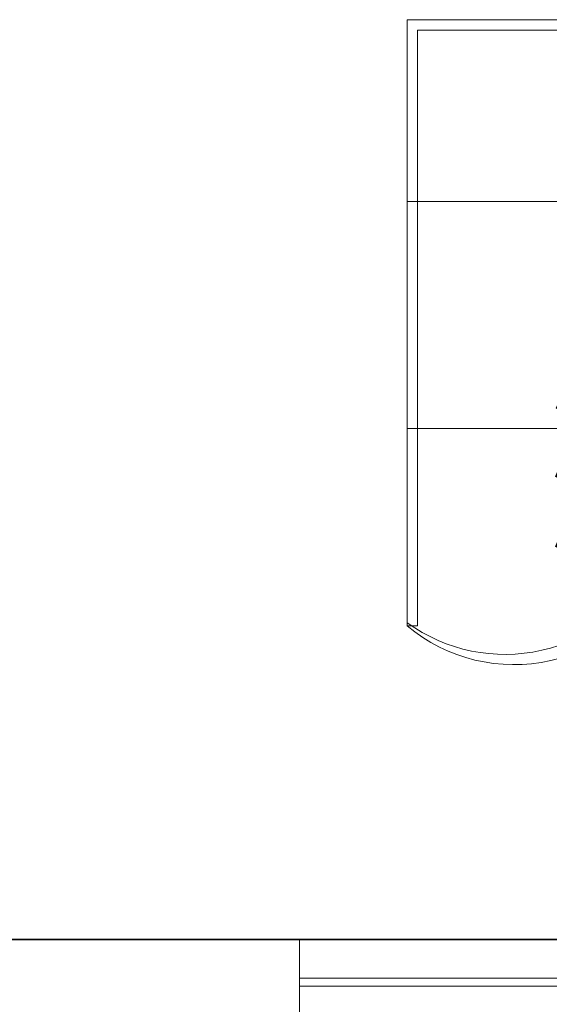
# Model space of a CAD drawing. Units: inches. Extents: x -61 to 1599, y -1316 to 257.
# Tile 159 of 204: x 1163 to 1214, y -1208 to -1113. Entities that reach past the tile are written whole.
import ezdxf

# ---------------------------------------------------------------- set-up
doc = ezdxf.new("R2010")
doc.units = ezdxf.units.IN
doc.header["$MEASUREMENT"] = 0
for name, color, linetype, lineweight in [('FURNITURE', 83, 'Continuous', 18), ('WALLS', 4, 'Continuous', 35), ('WINDOWS', 220, 'Continuous', 18)]:
    doc.layers.add(name, color=color, linetype=linetype, lineweight=lineweight)

# ---------------------------------------------------------------- blocks, each defined once
blk = doc.blocks.new('WIN-36IN-2')
for p, q in [((0, 9), (0, 0)), ((36, 9), (36, 0)), ((0, 5.262), (36, 5.262)), ((0, 4.5), (36, 4.5)), ((0, 4.5), (36, 4.5))]:
    blk.add_line(p, q)
blk = doc.blocks.new('MASTER-BEDROOM-CONSOLE')
for p, q in [((0, 44.886), (23.587, 44.886)), ((23.587, 37.779), (23.587, 9.438)), ((23.587, 37.779), (24.943, 35.589)), ((24.943, 35.589), (24.943, 9.456)), ((18.162, 33.228), (18.879, 30.704)), ((18.162, 33.228), (19.133, 31.826)), ((18.162, 33.228), (18.181, 31.167)), ((23.587, 30.804), (21.228, 29.654)), ((23.587, 30.804), (21.894, 30.592)), ((23.587, 30.804), (22.038, 29.443)), ((18.203, 28.51), (18.441, 28.869)), ((18.441, 28.869), (18.678, 29.228)), ((19.963, 28.553), (19.841, 28.966)), ((19.008, 27.84), (18.615, 28.016)), ((19.008, 27.84), (18.707, 27.533)), ((19.008, 27.84), (18.833, 27.448)), ((19.008, 27.84), (18.886, 28.253)), ((19.184, 28.233), (19.008, 27.84)), ((19.309, 28.148), (19.008, 27.84)), ((19.401, 27.665), (19.008, 27.84)), ((19.13, 27.428), (19.008, 27.84)), ((20.085, 28.141), (19.963, 28.553)), ((18.061, 27.072), (17.939, 27.485)), ((18.183, 26.66), (18.061, 27.072)), ((19.38, 26.517), (19.618, 26.876)), ((19.618, 26.876), (19.855, 27.235)), ((14.429, 24.877), (15.978, 26.238)), ((14.429, 24.877), (16.788, 26.026)), ((18.084, 26.588), (18.801, 24.064)), ((18.084, 26.588), (19.055, 25.186)), ((18.084, 26.588), (18.103, 24.527)), ((14.429, 24.877), (16.122, 25.089)), ((19.854, 22.452), (19.137, 24.976)), ((19.854, 22.452), (19.835, 24.514)), ((23.509, 24.163), (21.15, 23.014)), ((23.509, 24.163), (21.816, 23.952)), ((23.509, 24.163), (21.96, 22.803)), ((19.854, 22.452), (18.883, 23.854)), ((0, 22.886), (23.587, 22.886)), ((18.125, 21.87), (18.362, 22.229)), ((18.362, 22.229), (18.6, 22.588)), ((19.885, 21.913), (19.763, 22.326)), ((18.93, 21.2), (18.537, 21.376)), ((18.93, 21.2), (18.629, 20.893)), ((18.93, 21.2), (18.754, 20.808)), ((18.93, 21.2), (18.808, 21.613)), ((19.105, 21.593), (18.93, 21.2)), ((19.23, 21.508), (18.93, 21.2)), ((19.322, 21.025), (18.93, 21.2)), ((19.052, 20.788), (18.93, 21.2)), ((20.007, 21.5), (19.885, 21.913)), ((17.983, 20.432), (17.861, 20.845)), ((18.105, 20.02), (17.983, 20.432)), ((19.302, 19.877), (19.54, 20.236)), ((19.54, 20.236), (19.777, 20.595)), ((14.351, 18.237), (15.9, 19.598)), ((14.351, 18.237), (16.71, 19.386)), ((18.084, 19.819), (18.801, 17.295)), ((18.084, 19.819), (19.055, 18.417)), ((18.084, 19.819), (18.103, 17.757)), ((14.351, 18.237), (16.043, 18.448)), ((19.776, 15.812), (19.059, 18.336)), ((19.776, 15.812), (18.804, 17.214)), ((19.776, 15.812), (19.757, 17.874)), ((23.509, 17.394), (21.15, 16.245)), ((23.509, 17.394), (21.816, 17.183)), ((23.509, 17.394), (21.96, 16.033)), ((18.125, 15.101), (18.362, 15.459)), ((18.362, 15.459), (18.6, 15.818)), ((19.885, 15.143), (19.763, 15.556)), ((18.93, 14.431), (18.537, 14.606)), ((18.93, 14.431), (18.629, 14.123)), ((18.93, 14.431), (18.754, 14.038)), ((18.93, 14.431), (18.808, 14.843)), ((19.105, 14.823), (18.93, 14.431)), ((19.23, 14.738), (18.93, 14.431)), ((19.322, 14.255), (18.93, 14.431)), ((19.052, 14.018), (18.93, 14.431)), ((20.007, 14.731), (19.885, 15.143)), ((17.983, 13.663), (17.861, 14.075)), ((18.105, 13.25), (17.983, 13.663)), ((19.302, 13.108), (19.54, 13.466)), ((19.54, 13.466), (19.777, 13.825)), ((14.351, 11.468), (15.9, 12.828)), ((14.351, 11.468), (16.71, 12.617)), ((14.351, 11.468), (16.043, 11.679)), ((19.776, 9.043), (19.059, 11.567)), ((19.776, 9.043), (19.757, 11.104)), ((19.776, 9.043), (18.804, 10.445)), ((22.587, 9.438), (23.587, 9.438)), ((1, 3.748), (0, 3.748))]:
    blk.add_line(p, q)
for points in [[(0, 3.748), (0, 62.524), (23.587, 62.524), (23.587, 9.438)], [(1, 3.748), (1, 61.524), (22.587, 61.524), (22.587, 9.438)]]:
    blk.add_lwpolyline(points)
for points in [[(14.429, 24.877), (18.162, 33.228), (23.587, 30.804), (19.854, 22.452)], [(14.351, 18.237), (18.084, 26.588), (23.509, 24.163), (19.776, 15.812)], [(14.351, 11.468), (18.084, 19.819), (23.509, 17.394), (19.776, 9.043)]]:
    blk.add_lwpolyline(points, close=True)
for centre, radius in [((19.008, 27.84), 0.567), ((19.008, 27.84), 0.567), ((19.008, 27.84), 0.43), ((18.93, 21.2), 0.567), ((18.93, 21.2), 0.567), ((18.93, 21.2), 0.43), ((18.93, 14.431), 0.567), ((18.93, 14.431), 0.567), ((18.93, 14.431), 0.43)]:
    blk.add_circle(centre, radius)
for centre, radius, start, end in [((0.46, 36.131), 17.938, 321.14464, 350.6879), ((24.495, 40.115), 9.356, 227.40134, 264.43121), ((19.167, 31.62), 0.209, 99.3213, 167.2974), ((18.925, 31.877), 0.214, 280.21251, 346.40619), ((19.095, 32.037), 0.214, 280.21251, 346.40619), ((19.338, 31.78), 0.209, 99.3213, 167.2974), ((18.215, 30.96), 0.209, 99.3213, 167.2974), ((17.973, 31.217), 0.214, 280.21251, 346.40619), ((18.143, 31.378), 0.214, 280.21251, 346.40619), ((18.385, 31.121), 0.209, 99.3213, 167.2974), ((18.913, 30.498), 0.209, 99.3213, 167.2974), ((18.67, 30.755), 0.214, 280.21251, 346.40619), ((18.841, 30.915), 0.214, 280.21251, 346.40619), ((19.083, 30.658), 0.209, 99.3213, 167.2974), ((37.556, 19.55), 17.938, 141.14464, 170.6879), ((22.071, 30.471), 0.214, 145.42636, 211.62004), ((22.077, 30.705), 0.214, 145.42636, 211.62004), ((21.718, 30.48), 0.209, 324.53515, 32.51125), ((21.724, 30.714), 0.209, 324.53515, 32.51125), ((21.405, 29.533), 0.214, 145.42636, 211.62004), ((21.411, 29.767), 0.214, 145.42636, 211.62004), ((21.052, 29.542), 0.209, 324.53515, 32.51125), ((21.058, 29.776), 0.209, 324.53515, 32.51125), ((22.221, 29.555), 0.214, 145.42636, 211.62004), ((21.867, 29.564), 0.209, 324.53515, 32.51125), ((22.215, 29.321), 0.214, 145.42636, 211.62004), ((21.861, 29.33), 0.209, 324.53515, 32.51125), ((0.382, 29.491), 17.938, 321.14464, 350.6879), ((16.149, 26.117), 0.209, 144.53515, 212.51125), ((16.155, 26.351), 0.209, 144.53515, 212.51125), ((15.796, 26.126), 0.214, 325.42636, 31.62004), ((15.802, 26.36), 0.214, 325.42636, 31.62004), ((16.959, 25.905), 0.209, 144.53515, 212.51125), ((16.965, 26.139), 0.209, 144.53515, 212.51125), ((16.605, 25.914), 0.214, 325.42636, 31.62004), ((16.611, 26.148), 0.214, 325.42636, 31.62004), ((24.416, 33.475), 9.356, 227.40134, 264.43121), ((13.521, 15.565), 9.356, 47.40134, 84.43121), ((16.292, 24.967), 0.209, 144.53515, 212.51125), ((16.298, 25.201), 0.209, 144.53515, 212.51125), ((15.939, 24.976), 0.214, 325.42636, 31.62004), ((15.945, 25.21), 0.214, 325.42636, 31.62004), ((19.089, 24.98), 0.209, 99.3213, 167.2974), ((18.847, 25.237), 0.214, 280.21251, 346.40619), ((19.175, 24.765), 0.214, 100.21251, 166.40619), ((18.933, 25.022), 0.209, 279.3213, 347.2974), ((19.017, 25.397), 0.214, 280.21251, 346.40619), ((19.259, 25.14), 0.209, 99.3213, 167.2974), ((19.103, 25.183), 0.209, 279.3213, 347.2974), ((19.346, 24.926), 0.214, 100.21251, 166.40619), ((18.137, 24.32), 0.209, 99.3213, 167.2974), ((17.894, 24.577), 0.214, 280.21251, 346.40619), ((18.065, 24.738), 0.214, 280.21251, 346.40619), ((18.307, 24.48), 0.209, 99.3213, 167.2974), ((18.834, 23.858), 0.209, 99.3213, 167.2974), ((18.592, 24.115), 0.214, 280.21251, 346.40619), ((18.763, 24.275), 0.214, 280.21251, 346.40619), ((19.005, 24.018), 0.209, 99.3213, 167.2974), ((18.849, 24.061), 0.209, 279.3213, 347.2974), ((19.091, 23.804), 0.214, 100.21251, 166.40619), ((19.873, 24.303), 0.214, 100.21251, 166.40619), ((19.631, 24.56), 0.209, 279.3213, 347.2974), ((37.478, 12.91), 17.938, 141.14464, 170.6879), ((19.801, 24.721), 0.209, 279.3213, 347.2974), ((20.043, 24.464), 0.214, 100.21251, 166.40619), ((21.993, 23.83), 0.214, 145.42636, 211.62004), ((21.999, 24.065), 0.214, 145.42636, 211.62004), ((21.64, 23.84), 0.209, 324.53515, 32.51125), ((21.646, 24.074), 0.209, 324.53515, 32.51125), ((18.921, 23.643), 0.214, 100.21251, 166.40619), ((18.678, 23.9), 0.209, 279.3213, 347.2974), ((21.326, 22.892), 0.214, 145.42636, 211.62004), ((21.332, 23.127), 0.214, 145.42636, 211.62004), ((20.973, 22.902), 0.209, 324.53515, 32.51125), ((20.979, 23.136), 0.209, 324.53515, 32.51125), ((22.142, 22.915), 0.214, 145.42636, 211.62004), ((21.789, 22.924), 0.209, 324.53515, 32.51125), ((22.136, 22.681), 0.214, 145.42636, 211.62004), ((21.783, 22.69), 0.209, 324.53515, 32.51125), ((0.382, 22.721), 17.938, 321.14464, 350.6879), ((16.07, 19.476), 0.209, 144.53515, 212.51125), ((16.076, 19.711), 0.209, 144.53515, 212.51125), ((15.717, 19.486), 0.214, 325.42636, 31.62004), ((15.723, 19.72), 0.214, 325.42636, 31.62004), ((16.88, 19.265), 0.209, 144.53515, 212.51125), ((16.886, 19.499), 0.209, 144.53515, 212.51125), ((16.527, 19.274), 0.214, 325.42636, 31.62004), ((16.533, 19.508), 0.214, 325.42636, 31.62004), ((24.416, 26.706), 9.356, 227.40134, 264.43121), ((13.443, 8.925), 9.356, 47.40134, 84.43121), ((16.214, 18.327), 0.209, 144.53515, 212.51125), ((16.22, 18.561), 0.209, 144.53515, 212.51125), ((15.861, 18.336), 0.214, 325.42636, 31.62004), ((15.867, 18.57), 0.214, 325.42636, 31.62004), ((19.089, 18.21), 0.209, 99.3213, 167.2974), ((18.847, 18.467), 0.214, 280.21251, 346.40619), ((19.097, 18.125), 0.214, 100.21251, 166.40619), ((18.855, 18.382), 0.209, 279.3213, 347.2974), ((19.017, 18.628), 0.214, 280.21251, 346.40619), ((19.259, 18.371), 0.209, 99.3213, 167.2974), ((19.025, 18.543), 0.209, 279.3213, 347.2974), ((19.267, 18.286), 0.214, 100.21251, 166.40619), ((18.137, 17.55), 0.209, 99.3213, 167.2974), ((17.894, 17.807), 0.214, 280.21251, 346.40619), ((18.065, 17.968), 0.214, 280.21251, 346.40619), ((18.307, 17.711), 0.209, 99.3213, 167.2974), ((18.834, 17.088), 0.209, 99.3213, 167.2974), ((18.592, 17.345), 0.214, 280.21251, 346.40619), ((18.842, 17.003), 0.214, 100.21251, 166.40619), ((18.6, 17.26), 0.209, 279.3213, 347.2974), ((18.763, 17.506), 0.214, 280.21251, 346.40619), ((19.005, 17.249), 0.209, 99.3213, 167.2974), ((18.771, 17.421), 0.209, 279.3213, 347.2974), ((19.013, 17.164), 0.214, 100.21251, 166.40619), ((19.795, 17.663), 0.214, 100.21251, 166.40619), ((19.552, 17.92), 0.209, 279.3213, 347.2974), ((19.723, 18.081), 0.209, 279.3213, 347.2974), ((19.965, 17.824), 0.214, 100.21251, 166.40619), ((37.478, 6.14), 17.938, 141.14464, 170.6879), ((21.993, 17.061), 0.214, 145.42636, 211.62004), ((21.999, 17.295), 0.214, 145.42636, 211.62004), ((21.64, 17.07), 0.209, 324.53515, 32.51125), ((21.646, 17.304), 0.209, 324.53515, 32.51125), ((21.326, 16.123), 0.214, 145.42636, 211.62004), ((21.332, 16.357), 0.214, 145.42636, 211.62004), ((20.973, 16.132), 0.209, 324.53515, 32.51125), ((20.979, 16.366), 0.209, 324.53515, 32.51125), ((22.142, 16.145), 0.214, 145.42636, 211.62004), ((21.789, 16.155), 0.209, 324.53515, 32.51125), ((22.136, 15.911), 0.214, 145.42636, 211.62004), ((21.783, 15.92), 0.209, 324.53515, 32.51125), ((16.07, 12.707), 0.209, 144.53515, 212.51125), ((16.076, 12.941), 0.209, 144.53515, 212.51125), ((15.717, 12.716), 0.214, 325.42636, 31.62004), ((15.723, 12.95), 0.214, 325.42636, 31.62004), ((16.88, 12.495), 0.209, 144.53515, 212.51125), ((16.886, 12.729), 0.209, 144.53515, 212.51125), ((16.527, 12.504), 0.214, 325.42636, 31.62004), ((16.533, 12.739), 0.214, 325.42636, 31.62004), ((13.443, 2.156), 9.356, 47.40134, 84.43121), ((16.214, 11.557), 0.209, 144.53515, 212.51125), ((16.22, 11.791), 0.209, 144.53515, 212.51125), ((15.861, 11.566), 0.214, 325.42636, 31.62004), ((15.867, 11.801), 0.214, 325.42636, 31.62004), ((19.097, 11.356), 0.214, 100.21251, 166.40619), ((18.855, 11.613), 0.209, 279.3213, 347.2974), ((19.025, 11.773), 0.209, 279.3213, 347.2974), ((19.267, 11.516), 0.214, 100.21251, 166.40619), ((18.771, 10.651), 0.209, 279.3213, 347.2974), ((19.013, 10.394), 0.214, 100.21251, 166.40619), ((19.795, 10.893), 0.214, 100.21251, 166.40619), ((19.552, 11.151), 0.209, 279.3213, 347.2974), ((19.723, 11.311), 0.209, 279.3213, 347.2974), ((19.965, 11.054), 0.214, 100.21251, 166.40619), ((18.842, 10.234), 0.214, 100.21251, 166.40619), ((18.6, 10.491), 0.209, 279.3213, 347.2974), ((10.308, 16.053), 16.053, 230.04489, 335.73444), ((9.449, 17.042), 16.053, 233.93821, 331.72641)]:
    blk.add_arc(centre, radius, start, end)
for points in [[(18.203, 28.51), (18.191, 28.604), (18.167, 28.791), (18.438, 28.884), (18.778, 28.897), (18.67, 29.157), (18.678, 29.228)], [(20.085, 28.141), (20.124, 28.226), (20.202, 28.398), (19.97, 28.566), (19.649, 28.679), (19.829, 28.896), (19.841, 28.966)], [(19.401, 27.665), (19.361, 27.75), (19.281, 27.921), (19.003, 27.854), (18.708, 27.683), (18.66, 27.961), (18.615, 28.016)], [(19.309, 28.148), (19.303, 28.054), (19.292, 27.866), (19.008, 27.825), (18.671, 27.876), (18.729, 27.6), (18.707, 27.533)], [(19.13, 27.428), (19.169, 27.514), (19.247, 27.685), (19.015, 27.854), (18.694, 27.966), (18.873, 28.183), (18.886, 28.253)], [(19.184, 28.233), (19.098, 28.193), (18.927, 28.113), (18.994, 27.835), (19.165, 27.54), (18.888, 27.492), (18.833, 27.448)], [(18.183, 26.66), (18.222, 26.746), (18.3, 26.917), (18.069, 27.086), (17.747, 27.198), (17.927, 27.415), (17.939, 27.485)], [(19.38, 26.517), (19.368, 26.611), (19.344, 26.798), (19.615, 26.891), (19.955, 26.904), (19.847, 27.164), (19.855, 27.235)], [(18.125, 21.87), (18.113, 21.964), (18.089, 22.151), (18.359, 22.244), (18.7, 22.257), (18.592, 22.517), (18.6, 22.588)], [(20.007, 21.5), (20.046, 21.586), (20.124, 21.758), (19.892, 21.926), (19.571, 22.039), (19.75, 22.256), (19.763, 22.326)], [(19.322, 21.025), (19.283, 21.11), (19.203, 21.281), (18.924, 21.214), (18.63, 21.043), (18.582, 21.321), (18.537, 21.376)], [(19.23, 21.508), (19.225, 21.414), (19.213, 21.226), (18.93, 21.185), (18.593, 21.236), (18.651, 20.96), (18.629, 20.893)], [(19.052, 20.788), (19.091, 20.874), (19.169, 21.045), (18.937, 21.214), (18.615, 21.326), (18.795, 21.543), (18.808, 21.613)], [(19.105, 21.593), (19.02, 21.553), (18.849, 21.473), (18.916, 21.195), (19.087, 20.9), (18.809, 20.852), (18.754, 20.808)], [(18.105, 20.02), (18.144, 20.105), (18.222, 20.277), (17.99, 20.445), (17.669, 20.558), (17.848, 20.775), (17.861, 20.845)], [(19.302, 19.877), (19.29, 19.971), (19.266, 20.158), (19.537, 20.251), (19.877, 20.264), (19.769, 20.524), (19.777, 20.595)], [(18.125, 15.101), (18.113, 15.194), (18.089, 15.381), (18.359, 15.474), (18.7, 15.488), (18.592, 15.748), (18.6, 15.818)], [(20.007, 14.731), (20.046, 14.817), (20.124, 14.988), (19.892, 15.157), (19.571, 15.269), (19.75, 15.486), (19.763, 15.556)], [(19.322, 14.255), (19.283, 14.341), (19.203, 14.511), (18.924, 14.445), (18.63, 14.274), (18.582, 14.551), (18.537, 14.606)], [(19.23, 14.738), (19.225, 14.644), (19.213, 14.456), (18.93, 14.416), (18.593, 14.466), (18.651, 14.191), (18.629, 14.123)], [(19.052, 14.018), (19.091, 14.104), (19.169, 14.276), (18.937, 14.444), (18.615, 14.557), (18.795, 14.773), (18.808, 14.843)], [(19.105, 14.823), (19.02, 14.784), (18.849, 14.704), (18.916, 14.425), (19.087, 14.131), (18.809, 14.083), (18.754, 14.038)], [(18.105, 13.25), (18.144, 13.336), (18.222, 13.508), (17.99, 13.676), (17.669, 13.788), (17.848, 14.005), (17.861, 14.075)], [(19.302, 13.108), (19.29, 13.201), (19.266, 13.388), (19.537, 13.481), (19.877, 13.495), (19.769, 13.755), (19.777, 13.825)]]:
    blk.add_open_spline(points, degree=3, knots=[0, 0, 0, 0, 0.249187, 0.498374, 0.766554, 1.034734, 1.034734, 1.034734, 1.034734])

msp = doc.modelspace()

# ---------------------------------------------------------------- linework, layer by layer
at = {"layer": 'WALLS'}
msp.add_line((1065.7028, -1202.169), (1215.7028, -1202.169), dxfattribs=at)

# ---------------------------------------------------------------- block references
at = {"layer": 'FURNITURE'}
msp.add_blockref('MASTER-BEDROOM-CONSOLE', (1200.602, -1175.5131), dxfattribs=at)
at = {"layer": 'WINDOWS'}
msp.add_blockref('WIN-36IN-2', (1190.158, -1211.1691), dxfattribs=at)

doc.saveas('drawing.dxf')
